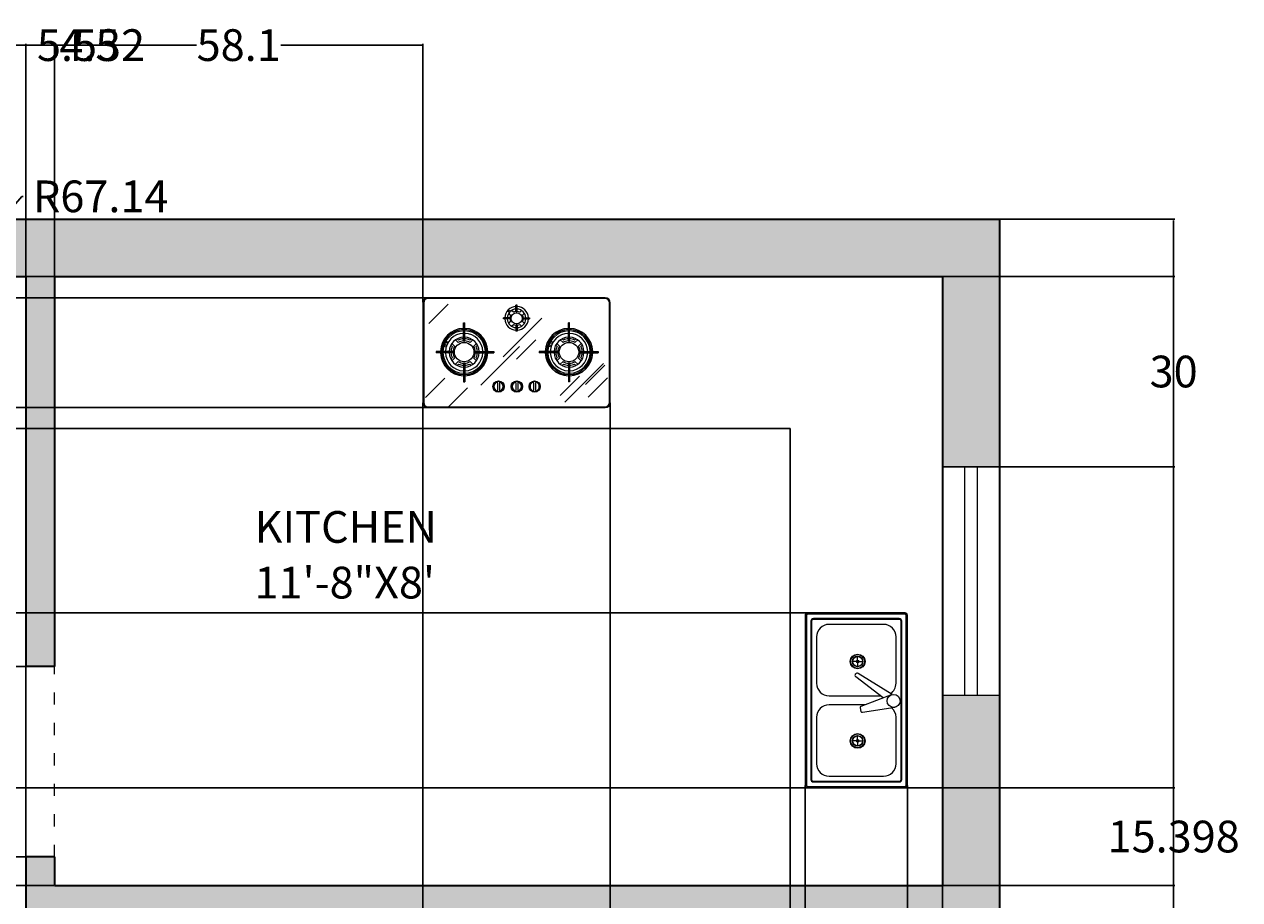
# Model space of a CAD drawing. Units: inches. Extents: x 2807 to 3326, y 2005 to 2580.
# Tile 12 of 12: x 3135 to 3326, y 2442 to 2580. Entities that reach past the tile are written whole.
import ezdxf

# ---------------------------------------------------------------- set-up
doc = ezdxf.new("R2010")
doc.units = ezdxf.units.IN
doc.header["$LTSCALE"] = 0.4
doc.linetypes.add('ACAD_ISO03W100', pattern=[30, 12, -18])
for name, color, linetype, lineweight in [('A-ANNO-DIMS', 2, 'Continuous', 18), ('A-AREA-IDEN', 5, 'Continuous', 18), ('A-DOOR-OVHD', 144, 'ACAD_ISO03W100', 18), ('A-EQPM', 8, 'Continuous', 18), ('A-FLOR-CASE', 233, 'Continuous', 25), ('A-FLOR-FIXT', 8, 'Continuous', 18), ('A-WALL-PATT', 231, 'Continuous', 13), ('WALL', 233, 'Continuous', 35), ('WINDOWS', 132, 'Continuous', 18)]:
    doc.layers.add(name, color=color, linetype=linetype, lineweight=lineweight)
doc.styles.get("Standard").update_dxf_attribs({"font": 'txt', "height": 5})
doc.dimstyles.get("Standard").update_dxf_attribs({"dimtxt": 0.18, "dimasz": 0.18, "dimexe": 0.18, "dimexo": 0.0625, "dimgap": 0.09, "dimtad": 0, "dimtih": 1, "dimtoh": 1, "dimdec": 4, "dimzin": 0, "dimdsep": 46, "dimtxsty": 'Standard', "dimcen": 0.09, "dimadec": 0, "dimazin": 0, "dimtfac": 1, "dimtdec": 4, "dimtofl": 0, "dimtmove": 0, "dimatfit": 3, "dimfxl": 1, "dimtolj": 1, "dimtzin": 0, "dimarcsym": 0})

# ---------------------------------------------------------------- blocks, each defined once
blk = doc.blocks.new('WIN-36')
at = {"ltscale": 0.4}
for p, q in [((0, 36), (0, 0)), ((9, 36), (0, 36)), ((3.5, 36), (3.5, 0)), ((5.5, 36), (5.5, 0)), ((9, 0), (9, 36)), ((0, 0), (9, 0))]:
    blk.add_line(p, q, dxfattribs=at)
blk = doc.blocks.new('*D32')
at = {"layer": 'A-ANNO-DIMS', "color": 0, "lineweight": -2, "ltscale": 0.4, "transparency": 16777216}
for p, q in [((3288.629691, 2549.576496), (3316.197191, 2549.576496)), ((3316.017191, 2549.396496), (3316.017191, 2295.416496)), ((3316.017191, 2036.256496), (3316.017191, 2290.236496)), ((3148.629691, 2036.076496), (3316.197191, 2036.076496))]:
    blk.add_line(p, q, dxfattribs=at)
at = {"layer": 'A-ANNO-DIMS', "color": 0, "ltscale": 0.4, "transparency": 16777216}
for points in [[(3315.987191, 2549.396496), (3316.047191, 2549.396496), (3316.017191, 2549.576496)], [(3315.987191, 2036.256496), (3316.047191, 2036.256496), (3316.017191, 2036.076496)]]:
    blk.add_solid(points, dxfattribs=at)
at = {"layer": 'Defpoints', "color": 0, "ltscale": 0.4, "transparency": 16777216}
for p in [(3288.567191, 2549.576496), (3316.017191, 2549.576496), (3148.567191, 2036.076496)]:
    blk.add_point(p, dxfattribs=at)
at = {"layer": 'A-ANNO-DIMS', "color": 0, "ltscale": 0.4, "transparency": 16777216, "insert": (3316.017191, 2292.826496), "char_height": 5, "attachment_point": 5}
blk.add_mtext('\\A1;513.5', dxfattribs=at)
blk = doc.blocks.new('*D48')
at = {"layer": 'A-ANNO-DIMS', "color": 0, "lineweight": -2, "ltscale": 0.4, "transparency": 16777216}
for p, q in [((3279.629691, 2540.576496), (3316.197191, 2540.576496)), ((3316.017191, 2540.396496), (3316.017191, 2528.166496)), ((3316.017191, 2510.756496), (3316.017191, 2522.986496)), ((3279.629691, 2510.576496), (3316.197191, 2510.576496))]:
    blk.add_line(p, q, dxfattribs=at)
at = {"layer": 'A-ANNO-DIMS', "color": 0, "ltscale": 0.4, "transparency": 16777216}
for points in [[(3315.987191, 2540.396496), (3316.047191, 2540.396496), (3316.017191, 2540.576496)], [(3315.987191, 2510.756496), (3316.047191, 2510.756496), (3316.017191, 2510.576496)]]:
    blk.add_solid(points, dxfattribs=at)
at = {"layer": 'Defpoints', "color": 0, "ltscale": 0.4, "transparency": 16777216}
for p in [(3279.567191, 2540.576496), (3316.017191, 2540.576496), (3279.567191, 2510.576496)]:
    blk.add_point(p, dxfattribs=at)
at = {"layer": 'A-ANNO-DIMS', "color": 0, "ltscale": 0.4, "transparency": 16777216, "insert": (3316.017191, 2525.576496), "char_height": 5, "attachment_point": 5}
blk.add_mtext('\\A1;30', dxfattribs=at)
blk = doc.blocks.new('*D49')
at = {"layer": 'A-ANNO-DIMS', "color": 0, "lineweight": -2, "ltscale": 0.4, "transparency": 16777216}
for p, q in [((3255.57, 2444.51), (3255.57, 2008.45)), ((3279.57, 2444.51), (3279.57, 2008.45)), ((3255.75, 2008.63), (3263.31, 2008.63)), ((3279.39, 2008.63), (3271.82, 2008.63))]:
    blk.add_line(p, q, dxfattribs=at)
at = {"layer": 'A-ANNO-DIMS', "color": 0, "ltscale": 0.4, "transparency": 16777216}
for points in [[(3255.75, 2008.66), (3255.75, 2008.6), (3255.57, 2008.63)], [(3279.39, 2008.66), (3279.39, 2008.6), (3279.57, 2008.63)]]:
    blk.add_solid(points, dxfattribs=at)
at = {"layer": 'Defpoints', "color": 0, "ltscale": 0.4, "transparency": 16777216}
for p in [(3255.57, 2444.58), (3279.57, 2444.58), (3279.57, 2008.63)]:
    blk.add_point(p, dxfattribs=at)
at = {"layer": 'A-ANNO-DIMS', "color": 0, "ltscale": 0.4, "transparency": 16777216, "insert": (3267.57, 2008.63), "char_height": 5, "attachment_point": 5}
blk.add_mtext('\\A1;24', dxfattribs=at)
blk = doc.blocks.new('*D50')
at = {"layer": 'A-ANNO-DIMS', "color": 0, "lineweight": -2, "ltscale": 0.4, "transparency": 16777216}
for p, q in [((3139.504691, 2540.576496), (2816.937191, 2540.576496)), ((2817.117191, 2540.396496), (2817.117191, 2531.166496)), ((2817.117191, 2516.756496), (2817.117191, 2525.986496)), ((3139.504691, 2516.576496), (2816.937191, 2516.576496))]:
    blk.add_line(p, q, dxfattribs=at)
at = {"layer": 'A-ANNO-DIMS', "color": 0, "ltscale": 0.4, "transparency": 16777216}
for points in [[(2817.087191, 2540.396496), (2817.147191, 2540.396496), (2817.117191, 2540.576496)], [(2817.087191, 2516.756496), (2817.147191, 2516.756496), (2817.117191, 2516.576496)]]:
    blk.add_solid(points, dxfattribs=at)
at = {"layer": 'Defpoints', "color": 0, "ltscale": 0.4, "transparency": 16777216}
for p in [(2817.117191, 2540.576496), (3139.567191, 2540.576496), (3139.567191, 2516.576496)]:
    blk.add_point(p, dxfattribs=at)
at = {"layer": 'A-ANNO-DIMS', "color": 0, "ltscale": 0.4, "transparency": 16777216, "insert": (2817.117191, 2528.576496), "char_height": 5, "attachment_point": 5}
blk.add_mtext('\\A1;24', dxfattribs=at)
blk = doc.blocks.new('*D51')
at = {"layer": 'A-ANNO-DIMS', "color": 0, "lineweight": -2, "ltscale": 0.4, "transparency": 16777216}
for p, q in [((3135.004691, 2479.076496), (2816.937191, 2479.076496)), ((2817.117191, 2478.896496), (2817.117191, 2466.666496)), ((2817.117191, 2449.256496), (2817.117191, 2461.486496)), ((3135.004691, 2449.076496), (2816.937191, 2449.076496))]:
    blk.add_line(p, q, dxfattribs=at)
at = {"layer": 'A-ANNO-DIMS', "color": 0, "ltscale": 0.4, "transparency": 16777216}
for points in [[(2817.087191, 2478.896496), (2817.147191, 2478.896496), (2817.117191, 2479.076496)], [(2817.087191, 2449.256496), (2817.147191, 2449.256496), (2817.117191, 2449.076496)]]:
    blk.add_solid(points, dxfattribs=at)
at = {"layer": 'Defpoints', "color": 0, "ltscale": 0.4, "transparency": 16777216}
for p in [(2817.117191, 2479.076496), (3135.067191, 2479.076496), (3135.067191, 2449.076496)]:
    blk.add_point(p, dxfattribs=at)
at = {"layer": 'A-ANNO-DIMS', "color": 0, "ltscale": 0.4, "transparency": 16777216, "insert": (2817.117191, 2464.076496), "char_height": 5, "attachment_point": 5}
blk.add_mtext('\\A1;30', dxfattribs=at)
blk = doc.blocks.new('*D53')
at = {"layer": 'A-ANNO-DIMS', "color": 0, "lineweight": -2, "ltscale": 0.4, "transparency": 16777216}
for p, q in [((3197.668377, 2520.617027), (3197.668377, 2008.446496)), ((3227.195877, 2520.617027), (3227.195877, 2008.446496)), ((3197.848377, 2008.626496), (3202.342127, 2008.626496)), ((3227.015877, 2008.626496), (3222.522127, 2008.626496))]:
    blk.add_line(p, q, dxfattribs=at)
at = {"layer": 'A-ANNO-DIMS', "color": 0, "ltscale": 0.4, "transparency": 16777216}
for points in [[(3197.848377, 2008.656496), (3197.848377, 2008.596496), (3197.668377, 2008.626496)], [(3227.015877, 2008.656496), (3227.015877, 2008.596496), (3227.195877, 2008.626496)]]:
    blk.add_solid(points, dxfattribs=at)
at = {"layer": 'Defpoints', "color": 0, "ltscale": 0.4, "transparency": 16777216}
for p in [(3197.668377, 2520.679527), (3227.195877, 2520.679527), (3227.195877, 2008.626496)]:
    blk.add_point(p, dxfattribs=at)
at = {"layer": 'A-ANNO-DIMS', "color": 0, "ltscale": 0.4, "transparency": 16777216, "insert": (3212.432127, 2008.626496), "char_height": 5, "attachment_point": 5}
blk.add_mtext('\\A1;29.53', dxfattribs=at)
blk = doc.blocks.new('*D54')
at = {"layer": 'A-ANNO-DIMS', "color": 0, "lineweight": -2, "ltscale": 0.4, "transparency": 16777216}
for p, q in [((3198.393277, 2537.214927), (2816.937191, 2537.214927)), ((2817.117191, 2537.034927), (2817.117191, 2531.143527)), ((2817.117191, 2520.072127), (2817.117191, 2525.963527)), ((3198.393277, 2519.892127), (2816.937191, 2519.892127))]:
    blk.add_line(p, q, dxfattribs=at)
at = {"layer": 'A-ANNO-DIMS', "color": 0, "ltscale": 0.4, "transparency": 16777216}
for points in [[(2817.087191, 2537.034927), (2817.147191, 2537.034927), (2817.117191, 2537.214927)], [(2817.087191, 2520.072127), (2817.147191, 2520.072127), (2817.117191, 2519.892127)]]:
    blk.add_solid(points, dxfattribs=at)
at = {"layer": 'Defpoints', "color": 0, "ltscale": 0.4, "transparency": 16777216}
for p in [(2817.117191, 2537.214927), (3198.455777, 2537.214927), (3198.455777, 2519.892127)]:
    blk.add_point(p, dxfattribs=at)
at = {"layer": 'A-ANNO-DIMS', "color": 0, "ltscale": 0.4, "transparency": 16777216, "insert": (2817.117191, 2528.553527), "char_height": 5, "attachment_point": 5}
blk.add_mtext('\\A1;17.323', dxfattribs=at)
blk = doc.blocks.new('*D55')
at = {"layer": 'A-ANNO-DIMS', "color": 0, "lineweight": -2, "ltscale": 0.4, "transparency": 16777216}
for p, q in [((3257.92, 2460.31), (3257.92, 2008.45)), ((3274.06, 2460.31), (3274.06, 2008.45)), ((3258.1, 2008.63), (3273.88, 2008.63)), ((3274.06, 2008.63), (3274.24, 2008.63))]:
    blk.add_line(p, q, dxfattribs=at)
at = {"layer": 'A-ANNO-DIMS', "color": 0, "ltscale": 0.4, "transparency": 16777216}
for points in [[(3258.1, 2008.66), (3258.1, 2008.6), (3257.92, 2008.63)], [(3273.88, 2008.66), (3273.88, 2008.6), (3274.06, 2008.63)]]:
    blk.add_solid(points, dxfattribs=at)
at = {"layer": 'Defpoints', "color": 0, "ltscale": 0.4, "transparency": 16777216}
for p in [(3257.92, 2460.37), (3274.06, 2460.37), (3274.06, 2008.63)]:
    blk.add_point(p, dxfattribs=at)
at = {"layer": 'A-ANNO-DIMS', "color": 0, "ltscale": 0.4, "transparency": 16777216, "insert": (3285.76, 2008.63), "char_height": 5, "attachment_point": 5}
blk.add_mtext('\\A1;16.142', dxfattribs=at)
blk = doc.blocks.new('*D56')
at = {"layer": 'A-ANNO-DIMS', "color": 0, "lineweight": -2, "ltscale": 0.4, "transparency": 16777216}
for p, q in [((3258.250937, 2487.533633), (2816.937191, 2487.533633)), ((2817.117191, 2487.353633), (2817.117191, 2476.344133)), ((2817.117191, 2460.154633), (2817.117191, 2471.164133)), ((3258.250937, 2459.974633), (2816.937191, 2459.974633))]:
    blk.add_line(p, q, dxfattribs=at)
at = {"layer": 'A-ANNO-DIMS', "color": 0, "ltscale": 0.4, "transparency": 16777216}
for points in [[(2817.087191, 2487.353633), (2817.147191, 2487.353633), (2817.117191, 2487.533633)], [(2817.087191, 2460.154633), (2817.147191, 2460.154633), (2817.117191, 2459.974633)]]:
    blk.add_solid(points, dxfattribs=at)
at = {"layer": 'Defpoints', "color": 0, "ltscale": 0.4, "transparency": 16777216}
for p in [(2817.117191, 2487.533633), (3258.313437, 2487.533633), (3258.313437, 2459.974633)]:
    blk.add_point(p, dxfattribs=at)
at = {"layer": 'A-ANNO-DIMS', "color": 0, "ltscale": 0.4, "transparency": 16777216, "insert": (2817.117191, 2473.754133), "char_height": 5, "attachment_point": 5}
blk.add_mtext('\\A1;27.56', dxfattribs=at)
blk = doc.blocks.new('*D57')
at = {"layer": 'A-ANNO-DIMS', "color": 0, "lineweight": -2, "ltscale": 0.4, "transparency": 16777216}
for p, q in [((3139.57, 2540.64), (3139.57, 2577.21)), ((3197.67, 2536.49), (3197.67, 2577.21)), ((3139.75, 2577.03), (3161.98, 2577.03)), ((3197.49, 2577.03), (3175.26, 2577.03))]:
    blk.add_line(p, q, dxfattribs=at)
at = {"layer": 'A-ANNO-DIMS', "color": 0, "ltscale": 0.4, "transparency": 16777216}
for points in [[(3139.75, 2577.06), (3139.75, 2577), (3139.57, 2577.03)], [(3197.49, 2577.06), (3197.49, 2577), (3197.67, 2577.03)]]:
    blk.add_solid(points, dxfattribs=at)
at = {"layer": 'Defpoints', "color": 0, "ltscale": 0.4, "transparency": 16777216}
for p in [(3197.67, 2577.03), (3139.57, 2540.58), (3197.67, 2536.43)]:
    blk.add_point(p, dxfattribs=at)
at = {"layer": 'A-ANNO-DIMS', "color": 0, "ltscale": 0.4, "transparency": 16777216, "insert": (3168.62, 2577.03), "char_height": 5, "attachment_point": 5}
blk.add_mtext('\\A1;58.1', dxfattribs=at)
blk = doc.blocks.new('*D58')
at = {"layer": 'A-ANNO-DIMS', "color": 0, "lineweight": -2, "ltscale": 0.4, "transparency": 16777216}
for p, q in [((3273.73, 2459.97), (3316.2, 2459.97)), ((3316.02, 2459.79), (3316.02, 2454.87)), ((3316.02, 2444.76), (3316.02, 2449.69)), ((3279.63, 2444.58), (3316.2, 2444.58))]:
    blk.add_line(p, q, dxfattribs=at)
at = {"layer": 'A-ANNO-DIMS', "color": 0, "ltscale": 0.4, "transparency": 16777216}
for points in [[(3315.99, 2459.79), (3316.05, 2459.79), (3316.02, 2459.97)], [(3315.99, 2444.76), (3316.05, 2444.76), (3316.02, 2444.58)]]:
    blk.add_solid(points, dxfattribs=at)
at = {"layer": 'Defpoints', "color": 0, "ltscale": 0.4, "transparency": 16777216}
for p in [(3273.67, 2459.97), (3316.02, 2459.97), (3279.57, 2444.58)]:
    blk.add_point(p, dxfattribs=at)
at = {"layer": 'A-ANNO-DIMS', "color": 0, "ltscale": 0.4, "transparency": 16777216, "insert": (3316.02, 2452.28), "char_height": 5, "attachment_point": 5}
blk.add_mtext('\\A1;15.398', dxfattribs=at)
blk = doc.blocks.new('*D66')
at = {"layer": 'A-ANNO-DIMS', "color": 0, "lineweight": -2, "ltscale": 0.4, "transparency": 16777216}
for p, q in [((3129.534988, 2263.581941), (3129.534988, 2577.206496)), ((3135.067191, 2275.138996), (3135.067191, 2577.206496)), ((3129.714988, 2577.026496), (3134.887191, 2577.026496)), ((3135.067191, 2577.026496), (3135.247191, 2577.026496))]:
    blk.add_line(p, q, dxfattribs=at)
at = {"layer": 'A-ANNO-DIMS', "color": 0, "ltscale": 0.4, "transparency": 16777216}
for points in [[(3129.714988, 2577.056496), (3129.714988, 2576.996496), (3129.534988, 2577.026496)], [(3134.887191, 2577.056496), (3134.887191, 2576.996496), (3135.067191, 2577.026496)]]:
    blk.add_solid(points, dxfattribs=at)
at = {"layer": 'Defpoints', "color": 0, "ltscale": 0.4, "transparency": 16777216}
for p in [(3135.067191, 2577.026496), (3135.067191, 2275.076496), (3129.534988, 2263.519441)]:
    blk.add_point(p, dxfattribs=at)
at = {"layer": 'A-ANNO-DIMS', "color": 0, "ltscale": 0.4, "transparency": 16777216, "insert": (3145.337191, 2577.026496), "char_height": 5, "attachment_point": 5}
blk.add_mtext('\\A1;5.532', dxfattribs=at)
blk = doc.blocks.new('*D70')
at = {"layer": 'A-ANNO-DIMS', "color": 0, "lineweight": -2, "ltscale": 0.4, "transparency": 16777216}
for p, q in [((3135.07, 2479.14), (3135.07, 2577.21)), ((3139.57, 2479.14), (3139.57, 2577.21)), ((3135.25, 2577.03), (3139.39, 2577.03)), ((3139.57, 2577.03), (3139.75, 2577.03))]:
    blk.add_line(p, q, dxfattribs=at)
at = {"layer": 'A-ANNO-DIMS', "color": 0, "ltscale": 0.4, "transparency": 16777216}
for points in [[(3135.25, 2577.06), (3135.25, 2577), (3135.07, 2577.03)], [(3139.39, 2577.06), (3139.39, 2577), (3139.57, 2577.03)]]:
    blk.add_solid(points, dxfattribs=at)
at = {"layer": 'Defpoints', "color": 0, "ltscale": 0.4, "transparency": 16777216}
for p in [(3139.57, 2577.03), (3135.07, 2479.08), (3139.57, 2479.08)]:
    blk.add_point(p, dxfattribs=at)
at = {"layer": 'A-ANNO-DIMS', "color": 0, "ltscale": 0.4, "transparency": 16777216, "insert": (3145.08, 2577.03), "char_height": 5, "attachment_point": 5}
blk.add_mtext('\\A1;4.5', dxfattribs=at)
blk = doc.blocks.new('*D71')
at = {"layer": 'A-ANNO-DIMS', "color": 0, "lineweight": -2, "ltscale": 0.4, "transparency": 16777216}
for p, q in [((3139.5, 2449.08), (2816.94, 2449.08)), ((2817.12, 2449.08), (2817.12, 2449.26)), ((2817.12, 2449.26), (2817.3, 2449.26)), ((2817.12, 2444.76), (2817.12, 2448.9)), ((3139.5, 2444.58), (2816.94, 2444.58))]:
    blk.add_line(p, q, dxfattribs=at)
at = {"layer": 'A-ANNO-DIMS', "color": 0, "ltscale": 0.4, "transparency": 16777216}
for points in [[(2817.09, 2448.9), (2817.15, 2448.9), (2817.12, 2449.08)], [(2817.09, 2444.76), (2817.15, 2444.76), (2817.12, 2444.58)]]:
    blk.add_solid(points, dxfattribs=at)
at = {"layer": 'Defpoints', "color": 0, "ltscale": 0.4, "transparency": 16777216}
for p in [(2817.12, 2449.08), (3139.57, 2449.08), (3139.57, 2444.58)]:
    blk.add_point(p, dxfattribs=at)
at = {"layer": 'A-ANNO-DIMS', "color": 0, "ltscale": 0.4, "transparency": 16777216, "insert": (2822.63, 2449.26), "char_height": 5, "attachment_point": 5}
blk.add_mtext('\\A1;4.5', dxfattribs=at)
blk = doc.blocks.new('*D75')
at = {"layer": 'A-ANNO-DIMS', "color": 0, "lineweight": -2, "ltscale": 0.4, "transparency": 16777216}
for p, q in [((3134.45, 2553.19), (3108.12, 2522.94)), ((3134.63, 2553.19), (3134.45, 2553.19)), ((3063.83, 2472.17), (3064.01, 2472.17)), ((3063.92, 2472.08), (3063.92, 2472.26))]:
    blk.add_line(p, q, dxfattribs=at)
at = {"layer": 'A-ANNO-DIMS', "color": 0, "ltscale": 0.4, "transparency": 16777216}
blk.add_solid([(3108.09, 2522.96), (3108.14, 2522.92), (3108, 2522.81)], dxfattribs=at)
at = {"layer": 'Defpoints', "color": 0, "ltscale": 0.4, "transparency": 16777216}
for p in [(3108, 2522.81), (3063.92, 2472.17)]:
    blk.add_point(p, dxfattribs=at)
at = {"layer": 'A-ANNO-DIMS', "color": 0, "ltscale": 0.4, "transparency": 16777216, "insert": (3146.86, 2553.19), "char_height": 5, "attachment_point": 5}
blk.add_mtext('\\A1;R67.14', dxfattribs=at)

msp = doc.modelspace()

# ---------------------------------------------------------------- hatches: boundary and pattern name
at = {"layer": 'A-WALL-PATT', "ltscale": 0.4}
h = msp.add_hatch(color=256, dxfattribs=at)
h.dxf.hatch_style = 1
h.paths.add_polyline_path([(3288.5672, 2549.5765), (2941.5672, 2549.5765), (2941.5672, 2540.5765), (2993.5672, 2540.5765), (2993.5672, 2489.5693), (2998.0672, 2489.5693), (2998.0672, 2540.5765), (3135.0672, 2540.5765), (3135.0672, 2479.0765), (3139.5672, 2479.0765), (3139.5672, 2540.5765), (3279.5672, 2540.5765), (3279.5672, 2510.5765), (3288.5672, 2510.5765)])
h.paths.add_polyline_path([(2905.5672, 2549.5765), (2844.5672, 2549.5765), (2844.5672, 2445.94), (2853.5672, 2445.94), (2853.5672, 2540.5765), (2905.5672, 2540.5765)])
h.paths.add_polyline_path([(2853.5672, 2409.94), (2844.5672, 2409.94), (2844.5672, 2371.3497), (2853.5672, 2371.3497), (2853.5672, 2380.0765), (2909.0672, 2380.0765), (2909.0672, 2384.5765), (2853.5672, 2384.5765)])
h.paths.add_polyline_path([(2998.0672, 2389.0765), (2993.5672, 2389.0765), (2993.5672, 2384.5765), (2939.0672, 2384.5765), (2939.0672, 2380.0765), (2943.5672, 2380.0765), (2943.5672, 2314.0765), (2948.0672, 2314.0765), (2948.0672, 2380.0765), (2998.0672, 2380.0765)])
h.paths.add_polyline_path([(2998.0672, 2471.8029), (2993.5672, 2471.8029), (2993.5672, 2425.0765), (2998.0672, 2425.0765)])
h.paths.add_polyline_path([(2953.0672, 2279.5765), (2948.0672, 2279.5765), (2948.0672, 2284.0765), (2943.5672, 2284.0765), (2943.5672, 2279.5765), (2853.5672, 2279.5765), (2853.5672, 2289.0663), (2844.5672, 2289.0663), (2844.5672, 2227.8961), (2853.5672, 2227.8961), (2853.5672, 2275.0765), (2953.0672, 2275.0765)])
h.paths.add_polyline_path([(2943.5672, 2332.0765), (2853.5672, 2332.0765), (2853.5672, 2347.3497), (2844.5672, 2347.3497), (2844.5672, 2313.0663), (2853.5672, 2313.0663), (2853.5672, 2327.5765), (2943.5672, 2327.5765)])
h.paths.add_polyline_path([(3144.0672, 2279.5765), (2993.5672, 2279.5765), (2989.0672, 2279.5765), (2989.0672, 2275.0765), (2993.5672, 2275.0765), (2993.5672, 2144.5765), (2984.5672, 2144.5765), (2984.5672, 2135.5765), (2993.5672, 2135.5765), (2993.5672, 2120.0765), (3036.5672, 2120.0765), (3036.5672, 2129.0765), (2998.0672, 2129.0765), (2998.0672, 2275.0765), (3135.0672, 2275.0765), (3135.0672, 2129.0765), (3096.5672, 2129.0765), (3096.5672, 2120.0765), (3139.5672, 2120.0765), (3139.5672, 2135.5765), (3148.5672, 2135.5765), (3148.5672, 2144.5765), (3139.5672, 2144.5765), (3139.5672, 2275.0765), (3144.0672, 2275.0765)])
h.paths.add_polyline_path([(2984.5672, 2144.5765), (2925.9914, 2144.5765), (2925.9914, 2135.5765), (2984.5672, 2135.5765)])
h.paths.add_polyline_path([(2889.9914, 2144.5765), (2853.5672, 2144.5765), (2853.5672, 2191.8961), (2844.5672, 2191.8961), (2844.5672, 2135.5765), (2889.9914, 2135.5765)])
h.paths.add_polyline_path([(3196.0672, 2144.5765), (3148.5672, 2144.5765), (3148.5672, 2135.5765), (3196.0672, 2135.5765)])
h.paths.add_polyline_path([(3288.5672, 2191.8265), (3279.5672, 2191.8265), (3279.5672, 2144.5765), (3232.0672, 2144.5765), (3232.0672, 2135.5765), (3288.5672, 2135.5765)])
h.paths.add_polyline_path([(3288.5672, 2292.8229), (3279.5672, 2292.8229), (3279.5672, 2291.4371), (3279.5672, 2279.5765), (3189.5672, 2279.5765), (3189.5672, 2293.0765), (3185.0672, 2293.0765), (3185.0672, 2279.5765), (3180.0672, 2279.5765), (3180.0672, 2275.0765), (3279.5672, 2275.0765), (3279.5672, 2227.8265), (3288.5672, 2227.8265)])
h.paths.add_polyline_path([(3288.5672, 2368.0765), (3279.5672, 2368.0765), (3279.5672, 2332.0765), (3174.0672, 2332.0765), (3174.0672, 2327.5765), (3185.0672, 2327.5765), (3189.5672, 2327.5765), (3279.5672, 2327.5765), (3279.5672, 2316.8229), (3288.5672, 2316.8229)])
h.paths.add_polyline_path([(3288.5672, 2474.5765), (3279.5672, 2474.5765), (3279.5672, 2444.5765), (3139.5672, 2444.5765), (3139.5672, 2449.0765), (3135.0672, 2449.0765), (3135.0672, 2327.5765), (3144.0672, 2327.5765), (3144.0672, 2332.0765), (3139.5672, 2332.0765), (3139.5672, 2440.0765), (3279.5672, 2440.0765), (3279.5672, 2404.0765), (3288.5672, 2404.0765)])

# ---------------------------------------------------------------- linework, layer by layer
at = {"layer": 'A-DOOR-OVHD', "ltscale": 0.4}
for p, q in [((3135.0672, 2449.0765), (3135.0672, 2479.0765)), ((3139.5672, 2449.0765), (3139.5672, 2479.0765))]:
    msp.add_line(p, q, dxfattribs=at)
at = {"layer": 'A-EQPM'}
for p, q in [((3226.4085, 2537.2149), (3198.4558, 2537.2149)), ((3226.4085, 2537.0968), (3198.4558, 2537.0968)), ((3197.6684, 2536.4275), (3197.6684, 2520.6795)), ((3197.7865, 2536.4275), (3197.7865, 2520.6795)), ((3198.6099, 2533.1506), (3201.6567, 2536.1974)), ((3211.9263, 2534.9105), (3211.6387, 2535.198)), ((3212.5306, 2536.0588), (3212.3337, 2536.0588)), ((3212.3337, 2535.0366), (3212.3337, 2536.0588)), ((3212.5306, 2535.0366), (3212.5306, 2536.0588)), ((3212.938, 2534.9105), (3213.2255, 2535.198)), ((3227.0778, 2520.6795), (3227.0778, 2536.4275)), ((3227.1959, 2520.6795), (3227.1959, 2536.4275)), ((3204.069, 2533.2755), (3204.2658, 2533.2755)), ((3204.069, 2530.4097), (3204.069, 2533.2755)), ((3204.2658, 2530.4097), (3204.2658, 2533.2755)), ((3210.3033, 2527.8713), (3216.397, 2533.965)), ((3210.3568, 2533.8608), (3210.3568, 2534.0576)), ((3211.3547, 2534.0576), (3210.3568, 2534.0576)), ((3211.3547, 2533.8608), (3210.3568, 2533.8608)), ((3211.4809, 2534.4651), (3211.1933, 2534.7526)), ((3211.1933, 2533.1658), (3211.4809, 2533.4534)), ((3213.3834, 2534.4651), (3213.6709, 2534.7526)), ((3213.6709, 2533.1658), (3213.3834, 2533.4534)), ((3213.5095, 2534.0576), (3214.4834, 2534.0576)), ((3213.5095, 2533.8608), (3214.4834, 2533.8608)), ((3214.4834, 2534.0576), (3214.4834, 2533.8608)), ((3220.7953, 2533.2755), (3220.5984, 2533.2755)), ((3220.5984, 2530.4097), (3220.5984, 2533.2755)), ((3220.7953, 2530.4097), (3220.7953, 2533.2755)), ((3211.6387, 2532.7204), (3211.9263, 2533.008)), ((3212.3337, 2532.8818), (3212.3337, 2531.9238)), ((3212.5306, 2531.9238), (3212.3337, 2531.9238)), ((3212.5306, 2532.8818), (3212.5306, 2531.9238)), ((3213.2255, 2532.7204), (3212.938, 2533.008)), ((3202.0729, 2529.7331), (3202.2786, 2529.5275)), ((3202.2421, 2530.0094), (3202.6676, 2529.5838)), ((3202.7988, 2530.5662), (3203.2244, 2530.1406)), ((3203.0751, 2530.7353), (3203.2808, 2530.5297)), ((3205.0541, 2530.5297), (3205.2597, 2530.7353)), ((3205.1104, 2530.1406), (3205.536, 2530.5662)), ((3205.6672, 2529.5838), (3206.0928, 2530.0094)), ((3206.0563, 2529.5275), (3206.2619, 2529.7331)), ((3206.807, 2523.4072), (3212.9006, 2529.5008)), ((3212.4012, 2527.522), (3215.448, 2530.5688)), ((3218.808, 2529.5275), (3218.6024, 2529.7331)), ((3219.197, 2529.5838), (3218.7715, 2530.0094)), ((3219.7538, 2530.1406), (3219.3283, 2530.5662)), ((3219.8102, 2530.5297), (3219.6045, 2530.7353)), ((3221.7891, 2530.7353), (3221.5835, 2530.5297)), ((3222.0654, 2530.5662), (3221.6399, 2530.1406)), ((3222.6222, 2530.0094), (3222.1967, 2529.5838)), ((3222.7913, 2529.7331), (3222.5857, 2529.5275)), ((3202.5953, 2528.7392), (3199.7617, 2528.7392)), ((3199.7617, 2528.7392), (3199.7617, 2528.5424)), ((3202.5953, 2528.5424), (3199.7617, 2528.5424)), ((3202.0729, 2527.5485), (3202.2786, 2527.7542)), ((3202.2421, 2527.2722), (3202.6676, 2527.6978)), ((3205.6672, 2527.6978), (3206.0928, 2527.2722)), ((3205.9363, 2528.7392), (3208.8487, 2528.7392)), ((3205.9363, 2528.5424), (3208.8487, 2528.5424)), ((3206.0563, 2527.7542), (3206.2619, 2527.5485)), ((3208.8487, 2528.7392), (3208.8487, 2528.5424)), ((3216.0156, 2528.7392), (3216.0156, 2528.5424)), ((3218.9279, 2528.7392), (3216.0156, 2528.7392)), ((3218.9279, 2528.5424), (3216.0156, 2528.5424)), ((3218.808, 2527.7542), (3218.6024, 2527.5485)), ((3219.197, 2527.6978), (3218.7715, 2527.2722)), ((3222.6222, 2527.2722), (3222.1967, 2527.6978)), ((3222.4658, 2528.7392), (3225.2994, 2528.7392)), ((3222.4658, 2528.5424), (3225.2994, 2528.5424)), ((3222.7913, 2527.5485), (3222.5857, 2527.7542)), ((3225.2994, 2528.7392), (3225.2994, 2528.5424)), ((3202.7988, 2526.7155), (3203.2244, 2527.141)), ((3203.0751, 2526.5463), (3203.2808, 2526.752)), ((3204.069, 2526.8719), (3204.069, 2523.9761)), ((3204.2658, 2526.8719), (3204.2658, 2523.9761)), ((3205.0541, 2526.752), (3205.2597, 2526.5463)), ((3205.1104, 2527.141), (3205.536, 2526.7155)), ((3219.7538, 2527.141), (3219.3283, 2526.7155)), ((3219.8102, 2526.752), (3219.6045, 2526.5463)), ((3220.0155, 2520.7676), (3226.1091, 2526.8612)), ((3220.5984, 2526.8719), (3220.5984, 2523.9761)), ((3220.7953, 2526.8719), (3220.7953, 2523.9761)), ((3221.7891, 2526.5463), (3221.5835, 2526.752)), ((3222.0654, 2526.7155), (3221.6399, 2527.141)), ((3223.2788, 2523.5209), (3226.3256, 2526.5677)), ((3198.066, 2521.5051), (3201.1128, 2524.5519)), ((3204.069, 2523.9761), (3204.2658, 2523.9761)), ((3209.4259, 2523.8202), (3209.4259, 2522.61)), ((3209.7409, 2523.8202), (3209.7409, 2522.61)), ((3212.3133, 2523.8202), (3212.3133, 2522.61)), ((3212.6283, 2523.8202), (3212.6283, 2522.61)), ((3215.1234, 2523.8202), (3215.1234, 2522.61)), ((3215.4383, 2523.8202), (3215.4383, 2522.61)), ((3219.3162, 2521.7768), (3222.363, 2524.8237)), ((3220.7953, 2523.9761), (3220.5984, 2523.9761)), ((3223.7061, 2521.5439), (3226.7529, 2524.5907)), ((3201.6401, 2519.9524), (3204.6869, 2522.9992)), ((3198.4558, 2520.0102), (3226.4085, 2520.0102)), ((3198.4558, 2519.8921), (3226.4085, 2519.8921))]:
    msp.add_line(p, q, dxfattribs=at)
for centre, radius in [((3211.2874, 2535.1003), 0.147), ((3212.4321, 2533.9592), 0.8805), ((3201.1774, 2529.6675), 0.147), ((3201.396, 2530.1862), 0.147), ((3204.1674, 2528.6408), 1.5354), ((3217.7086, 2529.6402), 0.147), ((3217.9272, 2530.1589), 0.147), ((3220.6968, 2528.6408), 1.5354), ((3209.5834, 2523.2151), 0.8858), ((3209.5834, 2523.2151), 0.8465), ((3212.4708, 2523.2151), 0.8858), ((3212.4708, 2523.2151), 0.8465), ((3215.2809, 2523.2151), 0.8858), ((3215.2809, 2523.2151), 0.8465)]:
    msp.add_circle(centre, radius, dxfattribs=at)
for centre, radius, start, end in [((3198.4558, 2536.4275), 0.7874, 90, 180), ((3198.4558, 2536.4275), 0.6693, 90, 180), ((3226.4085, 2536.4275), 0.7874, 0, 90), ((3226.4085, 2536.4275), 0.6693, 0, 90), ((3212.4321, 2533.9592), 1.8648, 93.025523, 176.974477), ((3212.4321, 2533.9592), 1.4711, 93.836312, 176.163688), ((3212.4321, 2533.9592), 1.0774, 95.202979, 118.002104), ((3212.4321, 2535.0503), 0.0994, 187.950532, 352.049468), ((3212.4321, 2533.9592), 1.0774, 61.997896, 84.797021), ((3212.4321, 2533.9592), 1.8648, 3.025523, 86.974477), ((3212.4321, 2533.9592), 1.4711, 3.836312, 86.163688), ((3212.4321, 2533.9592), 1.8648, 183.025523, 266.974477), ((3212.4321, 2533.9592), 1.4711, 183.836312, 266.163688), ((3211.3235, 2533.9592), 0.1033, 287.631775, 72.368225), ((3212.4321, 2533.9592), 1.0774, 151.997896, 174.838362), ((3212.4321, 2533.9592), 1.0774, 185.161638, 208.002104), ((3212.4321, 2533.9592), 1.8648, 273.025523, 356.974477), ((3212.4321, 2533.9592), 1.4711, 273.836312, 356.163688), ((3212.4321, 2533.9592), 1.0774, 5.206014, 28.002104), ((3212.4321, 2533.9592), 1.0774, 331.997896, 354.793986), ((3213.522, 2533.9592), 0.0992, 97.223613, 262.776387), ((3204.1674, 2528.6408), 3.7401, 91.591754, 178.408246), ((3204.1674, 2528.6408), 3.5433, 91.591754, 178.408246), ((3204.1674, 2528.6408), 3.3464, 91.685413, 178.314587), ((3204.1674, 2528.6408), 2.9527, 91.910213, 178.089787), ((3204.1674, 2528.6408), 3.5433, 1.591754, 88.408246), ((3204.1674, 2528.6408), 3.3464, 1.685413, 88.314587), ((3204.1674, 2528.6408), 2.9527, 1.910213, 88.089787), ((3204.1674, 2528.6408), 3.7401, 1.591754, 88.408246), ((3212.4321, 2533.9592), 1.0774, 241.997896, 264.756927), ((3212.4321, 2532.8847), 0.0985, 358.331725, 181.668275), ((3212.4321, 2533.9592), 1.0774, 275.243073, 298.002104), ((3220.6968, 2528.6408), 3.7401, 91.591754, 178.408246), ((3220.6968, 2528.6408), 3.5433, 91.591754, 178.408246), ((3220.6968, 2528.6408), 3.3464, 91.685413, 178.314587), ((3220.6968, 2528.6408), 2.9527, 91.910213, 178.089787), ((3220.6968, 2528.6408), 3.5433, 1.591754, 88.408246), ((3220.6968, 2528.6408), 3.3464, 1.685413, 88.314587), ((3220.6968, 2528.6408), 2.9527, 1.910213, 88.089787), ((3220.6968, 2528.6408), 3.7401, 1.591754, 88.408246), ((3204.1674, 2528.6408), 2.3622, 92.388015, 177.611985), ((3204.1674, 2528.6408), 2.0866, 154.853885, 177.296366), ((3204.1674, 2528.6408), 1.7716, 147.839588, 176.815261), ((3204.1674, 2528.6408), 1.7716, 93.184739, 122.160412), ((3204.1674, 2528.6408), 2.0866, 92.703634, 115.146115), ((3204.1674, 2530.4214), 0.0991, 186.735374, 353.264626), ((3204.1674, 2528.6408), 2.3622, 2.388015, 87.611985), ((3204.1674, 2528.6408), 2.0866, 64.853885, 87.296366), ((3204.1674, 2528.6408), 1.7716, 57.839588, 86.815261), ((3204.1674, 2528.6408), 1.7716, 3.184739, 32.160412), ((3204.1674, 2528.6408), 2.0866, 2.703634, 25.146115), ((3220.6968, 2528.6408), 2.3622, 92.388015, 177.611985), ((3220.6968, 2528.6408), 2.0866, 154.853885, 177.296366), ((3220.6968, 2528.6408), 1.7716, 147.839588, 176.815261), ((3220.6968, 2528.6408), 1.7716, 93.184739, 122.160412), ((3220.6968, 2528.6408), 2.0866, 92.703634, 115.146115), ((3220.6968, 2530.4165), 0.0987, 183.957935, 356.042065), ((3220.6968, 2528.6408), 2.3622, 2.388015, 87.611985), ((3220.6968, 2528.6408), 2.0866, 64.853885, 87.296366), ((3220.6968, 2528.6408), 1.7716, 57.839588, 86.815261), ((3220.6968, 2528.6408), 1.7716, 3.184739, 32.160412), ((3220.6968, 2528.6408), 2.0866, 2.703634, 25.146115), ((3204.1674, 2528.6408), 3.7401, 181.591754, 268.408246), ((3204.1674, 2528.6408), 3.5433, 181.591754, 268.408246), ((3204.1674, 2528.6408), 3.3464, 181.685413, 268.314587), ((3204.1674, 2528.6408), 2.9527, 181.910213, 268.089787), ((3204.1674, 2528.6408), 2.3622, 182.388015, 267.611985), ((3204.1674, 2528.6408), 2.0866, 182.703634, 205.146115), ((3202.3651, 2528.6408), 0.1039, 288.751046, 71.248954), ((3204.1674, 2528.6408), 1.7716, 183.184739, 212.160412), ((3204.1674, 2528.6408), 2.9527, 271.910213, 358.089787), ((3204.1674, 2528.6408), 2.3622, 272.388015, 357.611985), ((3204.1674, 2528.6408), 3.3464, 271.685413, 358.314587), ((3204.1674, 2528.6408), 3.5433, 271.591754, 358.408246), ((3204.1674, 2528.6408), 3.7401, 271.591754, 358.408246), ((3204.1674, 2528.6408), 1.7716, 327.839588, 356.815261), ((3205.9732, 2528.6408), 0.1051, 110.550693, 249.449307), ((3204.1674, 2528.6408), 2.0866, 334.853885, 357.296366), ((3220.6968, 2528.6408), 3.7401, 181.591754, 268.408246), ((3220.6968, 2528.6408), 3.5433, 181.591754, 268.408246), ((3220.6968, 2528.6408), 3.3464, 181.685413, 268.314587), ((3220.6968, 2528.6408), 2.9527, 181.910213, 268.089787), ((3220.6968, 2528.6408), 2.3622, 182.388015, 267.611985), ((3220.6968, 2528.6408), 2.0866, 182.703634, 205.146115), ((3218.8952, 2528.6408), 0.1037, 288.411971, 71.588029), ((3220.6968, 2528.6408), 1.7716, 183.184739, 212.160412), ((3220.6968, 2528.6408), 3.5433, 271.591754, 358.408246), ((3220.6968, 2528.6408), 3.3464, 271.685413, 358.314587), ((3220.6968, 2528.6408), 2.9527, 271.910213, 358.089787), ((3220.6968, 2528.6408), 2.3622, 272.388015, 357.611985), ((3220.6968, 2528.6408), 3.7401, 271.591754, 358.408246), ((3220.6968, 2528.6408), 1.7716, 327.839588, 356.815261), ((3222.4908, 2528.6408), 0.1016, 104.294479, 255.705521), ((3220.6968, 2528.6408), 2.0866, 334.853885, 357.296366), ((3204.1674, 2528.6408), 1.7716, 237.839588, 266.815261), ((3204.1674, 2528.6408), 2.0866, 244.853885, 267.296366), ((3204.1674, 2526.8326), 0.106, 21.788523, 158.211477), ((3204.1674, 2528.6408), 1.7716, 273.184739, 302.160412), ((3204.1674, 2528.6408), 2.0866, 272.703634, 295.146115), ((3220.6968, 2528.6408), 1.7716, 237.839588, 266.815261), ((3220.6968, 2528.6408), 2.0866, 244.853885, 267.296366), ((3220.6968, 2526.84), 0.1035, 17.941804, 162.058196), ((3220.6968, 2528.6408), 1.7716, 273.184739, 302.160412), ((3220.6968, 2528.6408), 2.0866, 272.703634, 295.146115), ((3209.5834, 2523.2151), 0.7283, 111.323686, 248.676314), ((3209.3472, 2523.8202), 0.0787, 0, 111.323686), ((3209.8196, 2523.8202), 0.0787, 68.676314, 180), ((3209.5834, 2523.2151), 0.7283, 291.323686, 68.676314), ((3212.4708, 2523.2151), 0.7283, 111.323686, 248.676314), ((3212.2346, 2523.8202), 0.0787, 0, 111.323686), ((3212.707, 2523.8202), 0.0787, 68.676314, 180), ((3212.4708, 2523.2151), 0.7283, 291.323686, 68.676314), ((3215.2809, 2523.2151), 0.7283, 111.323686, 248.676314), ((3215.0446, 2523.8202), 0.0787, 0, 111.323686), ((3215.5171, 2523.8202), 0.0787, 68.676314, 180), ((3215.2809, 2523.2151), 0.7283, 291.323686, 68.676314), ((3209.3472, 2522.61), 0.0787, 248.676314, 0), ((3209.8196, 2522.61), 0.0787, 180, 291.323686), ((3212.2346, 2522.61), 0.0787, 248.676314, 0), ((3212.707, 2522.61), 0.0787, 180, 291.323686), ((3215.0446, 2522.61), 0.0787, 248.676314, 0), ((3215.5171, 2522.61), 0.0787, 180, 291.323686), ((3198.4558, 2520.6795), 0.7874, 180, 270), ((3198.4558, 2520.6795), 0.6693, 180, 270), ((3226.4085, 2520.6795), 0.6693, 270, 0), ((3226.4085, 2520.6795), 0.7874, 270, 0)]:
    msp.add_arc(centre, radius, start, end, dxfattribs=at)
at = {"layer": 'A-FLOR-CASE'}
for p, q in [((3139.5672, 2516.5765), (3255.5672, 2516.5765)), ((3255.5672, 2516.5765), (3255.5672, 2444.5765))]:
    msp.add_line(p, q, dxfattribs=at)
at = {"layer": 'A-FLOR-FIXT'}
for p, q in [((3257.9197, 2487.1399), (3257.9197, 2460.3683)), ((3258.1166, 2487.1399), (3258.1166, 2460.3683)), ((3273.6677, 2487.5336), (3258.3134, 2487.5336)), ((3273.6677, 2487.3368), (3258.3134, 2487.3368)), ((3273.8646, 2460.3683), (3273.8646, 2487.1399)), ((3274.0614, 2460.3683), (3274.0614, 2487.1399)), ((3258.8252, 2486.2344), (3258.8252, 2461.2738)), ((3258.9434, 2486.2344), (3258.9434, 2461.2738)), ((3272.7622, 2486.6281), (3259.2189, 2486.6281)), ((3272.7622, 2486.51), (3259.2189, 2486.51)), ((3270.2819, 2485.7226), (3261.6993, 2485.7226)), ((3273.0378, 2461.2738), (3273.0378, 2486.2344)), ((3273.1559, 2461.2738), (3273.1559, 2486.2344)), ((3259.7308, 2483.7541), (3259.7308, 2476.4313)), ((3272.2504, 2476.4313), (3272.2504, 2483.7541)), ((3265.9983, 2479.8745), (3265.4078, 2479.8745)), ((3266.2022, 2480.0783), (3266.2022, 2480.6688)), ((3266.2022, 2479.6706), (3266.2022, 2479.0801)), ((3266.406, 2479.8745), (3266.9965, 2479.8745)), ((3265.8385, 2477.8963), (3265.8568, 2477.9211)), ((3271.6233, 2474.6518), (3266.2776, 2478.0012)), ((3270.2308, 2474.127), (3265.9, 2477.4599)), ((3261.6993, 2474.4628), (3269.7945, 2474.4628)), ((3271.6233, 2474.6518), (3266.7006, 2472.7966)), ((3267.3609, 2473.0455), (3261.6993, 2473.0455)), ((3266.5793, 2472.5637), (3266.7195, 2472.0148)), ((3266.94, 2471.8689), (3272.1327, 2472.6634)), ((3259.7308, 2471.077), (3259.7308, 2463.7542)), ((3272.2504, 2463.7542), (3272.2504, 2471.077)), ((3266.2022, 2467.5607), (3266.2022, 2468.1512)), ((3265.9983, 2467.3568), (3265.4078, 2467.3568)), ((3266.2022, 2467.1529), (3266.2022, 2466.5624)), ((3266.406, 2467.3568), (3266.9965, 2467.3568)), ((3259.2189, 2460.9983), (3272.7622, 2460.9983)), ((3259.2189, 2460.8801), (3272.7622, 2460.8801)), ((3261.6993, 2461.7857), (3270.2819, 2461.7857)), ((3258.3134, 2460.1715), (3273.6677, 2460.1715)), ((3258.3134, 2459.9746), (3273.6677, 2459.9746))]:
    msp.add_line(p, q, dxfattribs=at)
for centre, radius in [((3266.2022, 2479.8745), 1.162), ((3266.2022, 2479.8745), 1.0993), ((3266.2022, 2479.8745), 0.83), ((3266.2022, 2479.8745), 0.7944), ((3266.2022, 2479.8745), 0.2039), ((3266.2022, 2479.8745), 0.0958), ((3271.878, 2473.6576), 1.0263), ((3266.2022, 2467.3568), 1.162), ((3266.2022, 2467.3568), 1.0993), ((3266.2022, 2467.3568), 0.83), ((3266.2022, 2467.3568), 0.7944), ((3266.2022, 2467.3568), 0.2039), ((3266.2022, 2467.3568), 0.0958)]:
    msp.add_circle(centre, radius, dxfattribs=at)
for centre, radius, start, end in [((3258.3134, 2487.1399), 0.3937, 90, 180), ((3258.3134, 2487.1399), 0.1968, 90, 180), ((3273.6677, 2487.1399), 0.3937, 0, 90), ((3273.6677, 2487.1399), 0.1969, 0, 90), ((3259.2189, 2486.2344), 0.3937, 90, 180), ((3259.2189, 2486.2344), 0.2756, 90, 180), ((3261.6993, 2483.7541), 1.9685, 90, 180), ((3270.2819, 2483.7541), 1.9685, 0, 90), ((3272.7622, 2486.2344), 0.3937, 0, 90), ((3272.7622, 2486.2344), 0.2756, 0, 90), ((3266.0921, 2477.7095), 0.315, 143.630931, 232.418545), ((3266.1104, 2477.7343), 0.315, 57.930143, 143.630931), ((3261.6993, 2476.4313), 1.9685, 180, 270), ((3270.2819, 2476.4313), 1.9685, 304.086444, 0), ((3261.6993, 2471.077), 1.9685, 90, 180), ((3266.7701, 2472.6124), 0.1968, 110.649822, 194.323328), ((3266.9102, 2472.0635), 0.1968, 194.323328, 278.698535), ((3270.2819, 2471.077), 1.9685, 0, 49.57501), ((3261.6993, 2463.7542), 1.9685, 180, 270), ((3270.2819, 2463.7542), 1.9685, 270, 0), ((3258.3134, 2460.3683), 0.3937, 180, 270), ((3258.3134, 2460.3683), 0.1968, 180, 270), ((3259.2189, 2461.2738), 0.3937, 180, 270), ((3259.2189, 2461.2738), 0.2756, 180, 270), ((3272.7622, 2461.2738), 0.2756, 270, 0), ((3272.7622, 2461.2738), 0.3937, 270, 0), ((3273.6677, 2460.3683), 0.1969, 270, 0), ((3273.6677, 2460.3683), 0.3937, 270, 0)]:
    msp.add_arc(centre, radius, start, end, dxfattribs=at)
at = {"layer": 'WALL'}
for p, q in [((2844.5672, 2549.5765), (3288.5672, 2549.5765)), ((3288.5672, 2549.5765), (3288.5672, 2135.5765)), ((2998.0672, 2540.5765), (3135.0672, 2540.5765)), ((3135.0672, 2540.5765), (3135.0672, 2479.0765)), ((3139.5672, 2540.5765), (3139.5672, 2479.0765)), ((3139.5672, 2540.5765), (3279.5672, 2540.5765)), ((3279.5672, 2540.5765), (3279.5672, 2444.5765)), ((3139.5672, 2479.0765), (3135.0672, 2479.0765)), ((3139.5672, 2449.0765), (3135.0672, 2449.0765)), ((3135.0672, 2449.0765), (3135.0672, 2327.5765)), ((3139.5672, 2449.0765), (3139.5672, 2444.5765)), ((3139.5672, 2444.5765), (3279.5672, 2444.5765))]:
    msp.add_line(p, q, dxfattribs=at)

# ---------------------------------------------------------------- block references
at = {"layer": 'WINDOWS'}
msp.add_blockref('WIN-36', (3279.5672, 2474.5765), dxfattribs=at)

# ---------------------------------------------------------------- texts
at = {"layer": 'A-AREA-IDEN', "ltscale": 0.4}
for s, p in [('KITCHEN', (3171.1188, 2498.5804)), ('11\'-8"X8\'', (3171.1188, 2489.8065))]:
    msp.add_text(s, height=5, dxfattribs=at).set_placement(p)

# ---------------------------------------------------------------- dimensions: what is measured, and where the dimension line sits
at = {"layer": 'A-ANNO-DIMS', "ltscale": 0.4}
for base, p1, p2, override, picture, middle in [((3135.0672, 2577.0265), (3129.535, 2263.5194), (3135.0672, 2275.0765), {"dimdec": 3, "dimlfac": 1, "dimrnd": 0, "dimzin": 0, "dimdsep": 46, "dimlunit": 2}, '*D66', (3145.3372, 2577.0265)), ((3139.5672, 2577.0265), (3135.0672, 2479.0765), (3139.5672, 2479.0765), {"dimdec": 1, "dimlfac": 1, "dimrnd": 0, "dimzin": 0, "dimdsep": 46, "dimlunit": 2}, '*D70', (3145.0753, 2577.0265)), ((3197.6684, 2577.0265), (3139.5672, 2540.5765), (3197.6684, 2536.4275), {"dimdec": 1, "dimlfac": 1, "dimrnd": 0, "dimzin": 0, "dimdsep": 46, "dimlunit": 2}, '*D57', (3168.6178, 2577.0265)), ((3227.1959, 2008.6265), (3197.6684, 2520.6795), (3227.1959, 2520.6795), {"dimdec": 2, "dimlfac": 1, "dimrnd": 0, "dimzin": 0, "dimdsep": 46, "dimlunit": 2}, '*D53', (3212.4321, 2008.6265)), ((3274.0614, 2008.6265), (3257.9197, 2460.3683), (3274.0614, 2460.3683), {"dimdec": 3, "dimlfac": 1, "dimrnd": 0, "dimzin": 0, "dimdsep": 46, "dimlunit": 2}, '*D55', (3285.76, 2008.6265)), ((3279.5672, 2008.6265), (3255.5672, 2444.5765), (3279.5672, 2444.5765), {"dimdec": 0, "dimlfac": 1, "dimrnd": 0, "dimzin": 0, "dimdsep": 46, "dimlunit": 2}, '*D49', (3267.5672, 2008.6265))]:
    dim = msp.add_linear_dim(base=base, p1=p1, p2=p2, dimstyle='Standard', override=override, dxfattribs=at)
    dim.commit()
    dim.dimension.update_dxf_attribs({"geometry": picture, "text_midpoint": middle})
dim = msp.add_radius_dim(center=(3063.9187, 2472.1697), mpoint=(3107.9984, 2522.8081), dimstyle='Standard', override={"dimdec": 2, "dimlfac": 1, "dimrnd": 0, "dimzin": 0, "dimdsep": 46, "dimlunit": 2}, dxfattribs=at)
dim.commit()
dim.dimension.update_dxf_attribs({"geometry": '*D75', "text_midpoint": (3146.8591, 2553.1912), "dimtype": 164})
for base, p1, p2, override, picture, middle in [((3316.0172, 2549.5765), (3148.5672, 2036.0765), (3288.5672, 2549.5765), {"dimdec": 1, "dimlfac": 1, "dimrnd": 0, "dimzin": 0, "dimdsep": 46, "dimlunit": 2}, '*D32', (3316.0172, 2292.8265)), ((2817.1172, 2540.5765), (3139.5672, 2516.5765), (3139.5672, 2540.5765), {"dimdec": 0, "dimlfac": 1, "dimrnd": 0, "dimzin": 0, "dimdsep": 46, "dimlunit": 2}, '*D50', (2817.1172, 2528.5765)), ((3316.0172, 2540.5765), (3279.5672, 2510.5765), (3279.5672, 2540.5765), {"dimdec": 0, "dimlfac": 1, "dimrnd": 0, "dimzin": 0, "dimdsep": 46, "dimlunit": 2}, '*D48', (3316.0172, 2525.5765)), ((2817.1172, 2537.2149), (3198.4558, 2519.8921), (3198.4558, 2537.2149), {"dimdec": 3, "dimlfac": 1, "dimrnd": 0, "dimzin": 0, "dimdsep": 46, "dimlunit": 2}, '*D54', (2817.1172, 2528.5535)), ((2817.1172, 2487.5336), (3258.3134, 2459.9746), (3258.3134, 2487.5336), {"dimdec": 2, "dimlfac": 1, "dimrnd": 0, "dimzin": 0, "dimdsep": 46, "dimlunit": 2}, '*D56', (2817.1172, 2473.7541)), ((2817.1172, 2479.0765), (3135.0672, 2449.0765), (3135.0672, 2479.0765), {"dimdec": 0, "dimlfac": 1, "dimrnd": 0, "dimzin": 0, "dimdsep": 46, "dimlunit": 2}, '*D51', (2817.1172, 2464.0765)), ((3316.0172, 2459.9746), (3279.5672, 2444.5765), (3273.6677, 2459.9746), {"dimdec": 3, "dimlfac": 1, "dimrnd": 0, "dimzin": 0, "dimdsep": 46, "dimlunit": 2}, '*D58', (3316.0172, 2452.2756)), ((2817.1172, 2449.0765), (3139.5672, 2444.5765), (3139.5672, 2449.0765), {"dimdec": 1, "dimlfac": 1, "dimrnd": 0, "dimzin": 0, "dimdsep": 46, "dimlunit": 2}, '*D71', (2822.6253, 2449.2565))]:
    dim = msp.add_linear_dim(base=base, p1=p1, p2=p2, angle=90, dimstyle='Standard', override=override, dxfattribs=at)
    dim.commit()
    dim.dimension.update_dxf_attribs({"geometry": picture, "text_midpoint": middle})

doc.saveas('drawing.dxf')
